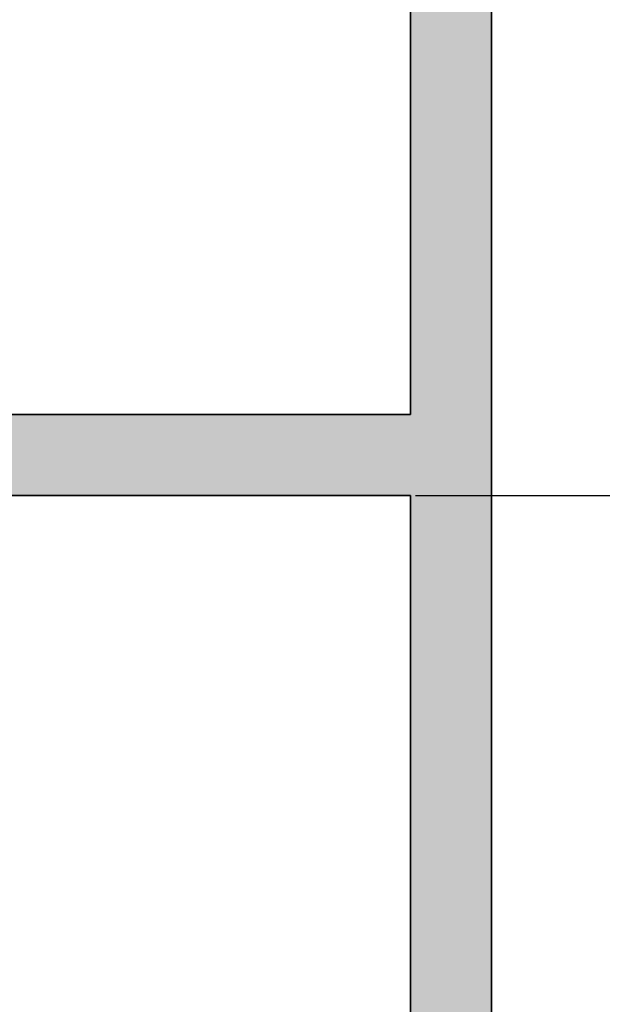
# Model space of a CAD drawing. Units: millimetres. Extents: x -22994 to 29398, y -19990 to 20176.
# Tile 38 of 135: x 183.3 to 190.48, y 41.76 to 53.9. Entities that reach past the tile are written whole.
import ezdxf
from ezdxf import colors
from ezdxf.entities.mleader import LeaderData, LeaderLine
from ezdxf.math import Vec2, Vec3

# ---------------------------------------------------------------- set-up
doc = ezdxf.new("R2010")
doc.units = ezdxf.units.MM
doc.header["$MEASUREMENT"] = 0
for name, color, linetype, lineweight in [('M-ANNO-TEXT', 7, 'Continuous', 25), ('M-DIMS', 2, 'Continuous', 18), ('M-EQPM-PATT', 7, 'Continuous', 18), ('M-PIPE', 7, 'Continuous', 35)]:
    doc.layers.add(name, color=color, linetype=linetype, lineweight=lineweight)
doc.styles.get("Standard").update_dxf_attribs({"font": 'arial.ttf'})
doc.dimstyles.get("Standard").update_dxf_attribs({"dimtxt": 0.18, "dimasz": 10000, "dimexe": 0.18, "dimexo": 0.0625, "dimgap": 0.09, "dimtad": 0, "dimtih": 1, "dimtoh": 1, "dimdec": 0, "dimzin": 0, "dimdsep": 46, "dimtxsty": 'Standard', "dimcen": 0.09, "dimadec": 0, "dimazin": 0, "dimtfac": 1, "dimtdec": 0, "dimtofl": 0, "dimtmove": 0, "dimatfit": 3, "dimfxl": 1, "dimtolj": 1, "dimtzin": 0, "dimlwd": 30, "dimarcsym": 0})

# ---------------------------------------------------------------- blocks, each defined once
blk = doc.blocks.new('*D2')
at = {"layer": 'Defpoints', "color": 0, "transparency": 16777216}
for p in [(6.677, 10.271), (290.852, 10.271), (290.852, -5.079)]:
    blk.add_point(p, dxfattribs=at)
at = {"layer": 'M-DIMS', "color": 0, "lineweight": -2, "transparency": 16777216}
for p, q in [((6.677, 10.209), (6.677, -5.259)), ((290.852, 10.209), (290.852, -5.259))]:
    blk.add_line(p, q, dxfattribs=at)
at = {"layer": 'M-DIMS', "color": 0, "lineweight": 30, "transparency": 16777216}
for p, q in [((-9993.323, -5.079), (-19993.323, -5.079)), ((10290.852, -5.079), (20290.852, -5.079))]:
    blk.add_line(p, q, dxfattribs=at)
at = {"layer": 'M-DIMS', "color": 0, "transparency": 16777216}
for points in [[(-9993.323, 1661.588), (-9993.323, -1671.745), (6.677, -5.079)], [(10290.852, 1661.588), (10290.852, -1671.745), (290.852, -5.079)]]:
    blk.add_solid(points, dxfattribs=at)
at = {"layer": 'M-DIMS', "color": 0, "transparency": 16777216, "insert": (148.765, -5.079), "char_height": 0.18, "attachment_point": 5}
blk.add_mtext('\\A1;284.2', dxfattribs=at)
blk = doc.blocks.new('*D3')
at = {"layer": 'Defpoints', "color": 0, "transparency": 16777216}
for p in [(110.265, 204.165), (110.265, 176.366), (95.833, 127.967)]:
    blk.add_point(p, dxfattribs=at)
at = {"layer": 'M-DIMS', "color": 0, "lineweight": -2, "transparency": 16777216}
for p, q in [((95.833, 128.03), (95.833, 204.345)), ((110.265, 176.429), (110.265, 204.345))]:
    blk.add_line(p, q, dxfattribs=at)
at = {"layer": 'M-DIMS', "color": 0, "lineweight": 30, "transparency": 16777216}
for p, q in [((-9904.167, 204.165), (-19904.167, 204.165)), ((10110.265, 204.165), (20110.265, 204.165))]:
    blk.add_line(p, q, dxfattribs=at)
at = {"layer": 'M-DIMS', "color": 0, "transparency": 16777216}
for points in [[(-9904.167, 1870.832), (-9904.167, -1462.501), (95.833, 204.165)], [(10110.265, 1870.832), (10110.265, -1462.501), (110.265, 204.165)]]:
    blk.add_solid(points, dxfattribs=at)
at = {"layer": 'M-DIMS', "color": 0, "transparency": 16777216, "insert": (103.049, 204.165), "char_height": 0.18, "attachment_point": 5}
blk.add_mtext('\\A1;14.432', dxfattribs=at)
blk = doc.blocks.new('*D4')
at = {"layer": 'Defpoints', "color": 0, "transparency": 16777216}
for p in [(116.265, 204.165), (110.265, 176.366), (116.265, 176.366)]:
    blk.add_point(p, dxfattribs=at)
at = {"layer": 'M-DIMS', "color": 0, "lineweight": -2, "transparency": 16777216}
for p, q in [((110.265, 176.429), (110.265, 204.345)), ((116.265, 176.429), (116.265, 204.345))]:
    blk.add_line(p, q, dxfattribs=at)
at = {"layer": 'M-DIMS', "color": 0, "lineweight": 30, "transparency": 16777216}
for p, q in [((-9889.735, 204.165), (-19889.735, 204.165)), ((10116.265, 204.165), (20116.265, 204.165))]:
    blk.add_line(p, q, dxfattribs=at)
at = {"layer": 'M-DIMS', "color": 0, "transparency": 16777216}
for points in [[(-9889.735, 1870.832), (-9889.735, -1462.501), (110.265, 204.165)], [(10116.265, 1870.832), (10116.265, -1462.501), (116.265, 204.165)]]:
    blk.add_solid(points, dxfattribs=at)
at = {"layer": 'M-DIMS', "color": 0, "transparency": 16777216, "insert": (113.265, 204.165), "char_height": 0.18, "attachment_point": 5}
blk.add_mtext('\\A1;6', dxfattribs=at)
blk = doc.blocks.new('*D5')
at = {"layer": 'Defpoints', "color": 0, "transparency": 16777216}
for p in [(181.265, 204.165), (116.265, 176.366), (181.265, 176.366)]:
    blk.add_point(p, dxfattribs=at)
at = {"layer": 'M-DIMS', "color": 0, "lineweight": -2, "transparency": 16777216}
for p, q in [((116.265, 176.429), (116.265, 204.345)), ((181.265, 176.429), (181.265, 204.345))]:
    blk.add_line(p, q, dxfattribs=at)
at = {"layer": 'M-DIMS', "color": 0, "lineweight": 30, "transparency": 16777216}
for p, q in [((-9883.735, 204.165), (-19883.735, 204.165)), ((10181.265, 204.165), (20181.265, 204.165))]:
    blk.add_line(p, q, dxfattribs=at)
at = {"layer": 'M-DIMS', "color": 0, "transparency": 16777216}
for points in [[(-9883.735, 1870.832), (-9883.735, -1462.501), (116.265, 204.165)], [(10181.265, 1870.832), (10181.265, -1462.501), (181.265, 204.165)]]:
    blk.add_solid(points, dxfattribs=at)
at = {"layer": 'M-DIMS', "color": 0, "transparency": 16777216, "insert": (148.765, 204.165), "char_height": 0.18, "attachment_point": 5}
blk.add_mtext('\\A1;65', dxfattribs=at)
blk = doc.blocks.new('*D6')
at = {"layer": 'Defpoints', "color": 0, "transparency": 16777216}
for p in [(187.265, 204.165), (181.265, 176.366), (187.265, 176.366)]:
    blk.add_point(p, dxfattribs=at)
at = {"layer": 'M-DIMS', "color": 0, "lineweight": -2, "transparency": 16777216}
for p, q in [((181.265, 176.429), (181.265, 204.345)), ((187.265, 176.429), (187.265, 204.345))]:
    blk.add_line(p, q, dxfattribs=at)
at = {"layer": 'M-DIMS', "color": 0, "lineweight": 30, "transparency": 16777216}
for p, q in [((-9818.735, 204.165), (-19818.735, 204.165)), ((10187.265, 204.165), (20187.265, 204.165))]:
    blk.add_line(p, q, dxfattribs=at)
at = {"layer": 'M-DIMS', "color": 0, "transparency": 16777216}
for points in [[(-9818.735, 1870.832), (-9818.735, -1462.501), (181.265, 204.165)], [(10187.265, 1870.832), (10187.265, -1462.501), (187.265, 204.165)]]:
    blk.add_solid(points, dxfattribs=at)
at = {"layer": 'M-DIMS', "color": 0, "transparency": 16777216, "insert": (184.265, 204.165), "char_height": 0.18, "attachment_point": 5}
blk.add_mtext('\\A1;6', dxfattribs=at)
blk = doc.blocks.new('*D7')
at = {"layer": 'Defpoints', "color": 0, "transparency": 16777216}
for p in [(201.697, 204.165), (187.265, 176.366), (201.697, 127.967)]:
    blk.add_point(p, dxfattribs=at)
at = {"layer": 'M-DIMS', "color": 0, "lineweight": -2, "transparency": 16777216}
for p, q in [((187.265, 176.429), (187.265, 204.345)), ((201.697, 128.03), (201.697, 204.345))]:
    blk.add_line(p, q, dxfattribs=at)
at = {"layer": 'M-DIMS', "color": 0, "lineweight": 30, "transparency": 16777216}
for p, q in [((-9812.735, 204.165), (-19812.735, 204.165)), ((10201.697, 204.165), (20201.697, 204.165))]:
    blk.add_line(p, q, dxfattribs=at)
at = {"layer": 'M-DIMS', "color": 0, "transparency": 16777216}
for points in [[(-9812.735, 1870.832), (-9812.735, -1462.501), (187.265, 204.165)], [(10201.697, 1870.832), (10201.697, -1462.501), (201.697, 204.165)]]:
    blk.add_solid(points, dxfattribs=at)
at = {"layer": 'M-DIMS', "color": 0, "transparency": 16777216, "insert": (194.481, 204.165), "char_height": 0.18, "attachment_point": 5}
blk.add_mtext('\\A1;14.432', dxfattribs=at)
blk = doc.blocks.new('*D8')
at = {"layer": 'Defpoints', "color": 0, "transparency": 16777216}
for p in [(227.648, 204.165), (227.648, 146.73), (201.697, 127.967)]:
    blk.add_point(p, dxfattribs=at)
at = {"layer": 'M-DIMS', "color": 0, "lineweight": -2, "transparency": 16777216}
for p, q in [((201.697, 128.03), (201.697, 204.345)), ((227.648, 146.792), (227.648, 204.345))]:
    blk.add_line(p, q, dxfattribs=at)
at = {"layer": 'M-DIMS', "color": 0, "lineweight": 30, "transparency": 16777216}
for p, q in [((-9798.303, 204.165), (-19798.303, 204.165)), ((10227.648, 204.165), (20227.648, 204.165))]:
    blk.add_line(p, q, dxfattribs=at)
at = {"layer": 'M-DIMS', "color": 0, "transparency": 16777216}
for points in [[(-9798.303, 1870.832), (-9798.303, -1462.501), (201.697, 204.165)], [(10227.648, 1870.832), (10227.648, -1462.501), (227.648, 204.165)]]:
    blk.add_solid(points, dxfattribs=at)
at = {"layer": 'M-DIMS', "color": 0, "transparency": 16777216, "insert": (214.673, 204.165), "char_height": 0.18, "attachment_point": 5}
blk.add_mtext('\\A1;25.95', dxfattribs=at)
blk = doc.blocks.new('*D9')
at = {"layer": 'Defpoints', "color": 0, "transparency": 16777216}
for p in [(187.265, 176.366), (306.202, 176.366), (290.852, 10.271)]:
    blk.add_point(p, dxfattribs=at)
at = {"layer": 'M-DIMS', "color": 0, "lineweight": 30, "transparency": 16777216}
for p, q in [((306.202, 10176.366), (306.202, 20176.366)), ((306.202, -9989.729), (306.202, -19989.729))]:
    blk.add_line(p, q, dxfattribs=at)
at = {"layer": 'M-DIMS', "color": 0, "lineweight": -2, "transparency": 16777216}
for p, q in [((187.327, 176.366), (306.382, 176.366)), ((290.915, 10.271), (306.382, 10.271))]:
    blk.add_line(p, q, dxfattribs=at)
at = {"layer": 'M-DIMS', "color": 0, "transparency": 16777216}
for points in [[(-1360.465, 10176.366), (1972.869, 10176.366), (306.202, 176.366)], [(-1360.465, -9989.729), (1972.869, -9989.729), (306.202, 10.271)]]:
    blk.add_solid(points, dxfattribs=at)
at = {"layer": 'M-DIMS', "color": 0, "transparency": 16777216, "insert": (306.202, 93.319), "char_height": 0.18, "attachment_point": 5}
blk.add_mtext('\\A1;166.1', dxfattribs=at)
blk = doc.blocks.new('*D10')
at = {"layer": 'Defpoints', "color": 0, "transparency": 16777216}
for p in [(125.65, 136.071), (133.346, 136.071), (133.346, -5.079)]:
    blk.add_point(p, dxfattribs=at)
at = {"layer": 'M-DIMS', "color": 0, "lineweight": -2, "transparency": 16777216}
for p, q in [((125.65, 136.009), (125.65, -5.259)), ((133.346, 136.009), (133.346, -5.259))]:
    blk.add_line(p, q, dxfattribs=at)
at = {"layer": 'M-DIMS', "color": 0, "lineweight": 30, "transparency": 16777216}
for p, q in [((-9874.35, -5.079), (-19874.35, -5.079)), ((10133.346, -5.079), (20133.346, -5.079))]:
    blk.add_line(p, q, dxfattribs=at)
at = {"layer": 'M-DIMS', "color": 0, "transparency": 16777216}
for points in [[(-9874.35, 1661.588), (-9874.35, -1671.745), (125.65, -5.079)], [(10133.346, 1661.588), (10133.346, -1671.745), (133.346, -5.079)]]:
    blk.add_solid(points, dxfattribs=at)
at = {"layer": 'M-DIMS', "color": 0, "transparency": 16777216, "insert": (129.498, -5.079), "char_height": 0.18, "attachment_point": 5}
blk.add_mtext('\\A1;7.696', dxfattribs=at)
blk = doc.blocks.new('*D11')
at = {"layer": 'Defpoints', "color": 0, "transparency": 16777216}
for p in [(133.346, 136.071), (135.65, 136.071), (135.65, -5.079)]:
    blk.add_point(p, dxfattribs=at)
at = {"layer": 'M-DIMS', "color": 0, "lineweight": -2, "transparency": 16777216}
for p, q in [((133.346, 136.009), (133.346, -5.259)), ((135.65, 136.009), (135.65, -5.259))]:
    blk.add_line(p, q, dxfattribs=at)
at = {"layer": 'M-DIMS', "color": 0, "lineweight": 30, "transparency": 16777216}
for p, q in [((-9866.654, -5.079), (-19866.654, -5.079)), ((10135.65, -5.079), (20135.65, -5.079))]:
    blk.add_line(p, q, dxfattribs=at)
at = {"layer": 'M-DIMS', "color": 0, "transparency": 16777216}
for points in [[(-9866.654, 1661.588), (-9866.654, -1671.745), (133.346, -5.079)], [(10135.65, 1661.588), (10135.65, -1671.745), (135.65, -5.079)]]:
    blk.add_solid(points, dxfattribs=at)
at = {"layer": 'M-DIMS', "color": 0, "transparency": 16777216, "insert": (134.498, -5.079), "char_height": 0.18, "attachment_point": 5}
blk.add_mtext('\\A1;2.304', dxfattribs=at)
blk = doc.blocks.new('*D12')
at = {"layer": 'Defpoints', "color": 0, "transparency": 16777216}
for p in [(135.65, 136.071), (145.65, 136.071), (145.65, -5.079)]:
    blk.add_point(p, dxfattribs=at)
at = {"layer": 'M-DIMS', "color": 0, "lineweight": -2, "transparency": 16777216}
for p, q in [((135.65, 136.009), (135.65, -5.259)), ((145.65, 136.009), (145.65, -5.259))]:
    blk.add_line(p, q, dxfattribs=at)
at = {"layer": 'M-DIMS', "color": 0, "lineweight": 30, "transparency": 16777216}
for p, q in [((-9864.35, -5.079), (-19864.35, -5.079)), ((10145.65, -5.079), (20145.65, -5.079))]:
    blk.add_line(p, q, dxfattribs=at)
at = {"layer": 'M-DIMS', "color": 0, "transparency": 16777216}
for points in [[(-9864.35, 1661.588), (-9864.35, -1671.745), (135.65, -5.079)], [(10145.65, 1661.588), (10145.65, -1671.745), (145.65, -5.079)]]:
    blk.add_solid(points, dxfattribs=at)
at = {"layer": 'M-DIMS', "color": 0, "transparency": 16777216, "insert": (140.65, -5.079), "char_height": 0.18, "attachment_point": 5}
blk.add_mtext('\\A1;10', dxfattribs=at)
blk = doc.blocks.new('*D13')
at = {"layer": 'Defpoints', "color": 0, "transparency": 16777216}
for p in [(145.65, 136.071), (155.65, 136.071), (155.65, -5.079)]:
    blk.add_point(p, dxfattribs=at)
at = {"layer": 'M-DIMS', "color": 0, "lineweight": -2, "transparency": 16777216}
for p, q in [((145.65, 136.009), (145.65, -5.259)), ((155.65, 136.009), (155.65, -5.259))]:
    blk.add_line(p, q, dxfattribs=at)
at = {"layer": 'M-DIMS', "color": 0, "lineweight": 30, "transparency": 16777216}
for p, q in [((-9854.35, -5.079), (-19854.35, -5.079)), ((10155.65, -5.079), (20155.65, -5.079))]:
    blk.add_line(p, q, dxfattribs=at)
at = {"layer": 'M-DIMS', "color": 0, "transparency": 16777216}
for points in [[(-9854.35, 1661.588), (-9854.35, -1671.745), (145.65, -5.079)], [(10155.65, 1661.588), (10155.65, -1671.745), (155.65, -5.079)]]:
    blk.add_solid(points, dxfattribs=at)
at = {"layer": 'M-DIMS', "color": 0, "transparency": 16777216, "insert": (150.65, -5.079), "char_height": 0.18, "attachment_point": 5}
blk.add_mtext('\\A1;10', dxfattribs=at)
blk = doc.blocks.new('*D14')
at = {"layer": 'Defpoints', "color": 0, "transparency": 16777216}
for p in [(155.65, 136.071), (165.65, 136.071), (165.65, -5.079)]:
    blk.add_point(p, dxfattribs=at)
at = {"layer": 'M-DIMS', "color": 0, "lineweight": -2, "transparency": 16777216}
for p, q in [((155.65, 136.009), (155.65, -5.259)), ((165.65, 136.009), (165.65, -5.259))]:
    blk.add_line(p, q, dxfattribs=at)
at = {"layer": 'M-DIMS', "color": 0, "lineweight": 30, "transparency": 16777216}
for p, q in [((-9844.35, -5.079), (-19844.35, -5.079)), ((10165.65, -5.079), (20165.65, -5.079))]:
    blk.add_line(p, q, dxfattribs=at)
at = {"layer": 'M-DIMS', "color": 0, "transparency": 16777216}
for points in [[(-9844.35, 1661.588), (-9844.35, -1671.745), (155.65, -5.079)], [(10165.65, 1661.588), (10165.65, -1671.745), (165.65, -5.079)]]:
    blk.add_solid(points, dxfattribs=at)
at = {"layer": 'M-DIMS', "color": 0, "transparency": 16777216, "insert": (160.65, -5.079), "char_height": 0.18, "attachment_point": 5}
blk.add_mtext('\\A1;10', dxfattribs=at)
blk = doc.blocks.new('*D15')
at = {"layer": 'Defpoints', "color": 0, "transparency": 16777216}
for p in [(173.346, 154.788), (173.346, 136.071), (306.202, 136.071)]:
    blk.add_point(p, dxfattribs=at)
at = {"layer": 'M-DIMS', "color": 0, "lineweight": 30, "transparency": 16777216}
for p, q in [((306.202, 10154.788), (306.202, 20154.788)), ((306.202, -9863.929), (306.202, -19863.929))]:
    blk.add_line(p, q, dxfattribs=at)
at = {"layer": 'M-DIMS', "color": 0, "lineweight": -2, "transparency": 16777216}
for p, q in [((173.408, 154.788), (306.382, 154.788)), ((173.408, 136.071), (306.382, 136.071))]:
    blk.add_line(p, q, dxfattribs=at)
at = {"layer": 'M-DIMS', "color": 0, "transparency": 16777216}
for points in [[(-1360.465, 10154.788), (1972.869, 10154.788), (306.202, 154.788)], [(-1360.465, -9863.929), (1972.869, -9863.929), (306.202, 136.071)]]:
    blk.add_solid(points, dxfattribs=at)
at = {"layer": 'M-DIMS', "color": 0, "transparency": 16777216, "insert": (306.202, 145.43), "char_height": 0.18, "attachment_point": 5}
blk.add_mtext('\\A1;18.717', dxfattribs=at)
blk = doc.blocks.new('*D16')
at = {"layer": 'Defpoints', "color": 0, "transparency": 16777216}
for p in [(120.17, 204.165), (110.466, 48.035), (120.17, 48.035)]:
    blk.add_point(p, dxfattribs=at)
at = {"layer": 'M-DIMS', "color": 0, "lineweight": -2, "transparency": 16777216}
for p, q in [((110.466, 48.097), (110.466, 204.345)), ((120.17, 48.097), (120.17, 204.345))]:
    blk.add_line(p, q, dxfattribs=at)
at = {"layer": 'M-DIMS', "color": 0, "lineweight": 30, "transparency": 16777216}
for p, q in [((-9889.534, 204.165), (-19889.534, 204.165)), ((10120.17, 204.165), (20120.17, 204.165))]:
    blk.add_line(p, q, dxfattribs=at)
at = {"layer": 'M-DIMS', "color": 0, "transparency": 16777216}
for points in [[(-9889.534, 1870.832), (-9889.534, -1462.501), (110.466, 204.165)], [(10120.17, 1870.832), (10120.17, -1462.501), (120.17, 204.165)]]:
    blk.add_solid(points, dxfattribs=at)
at = {"layer": 'M-DIMS', "color": 0, "transparency": 16777216, "insert": (115.318, 204.165), "char_height": 0.18, "attachment_point": 5}
blk.add_mtext('\\A1;9.704', dxfattribs=at)
blk = doc.blocks.new('*D17')
at = {"layer": 'Defpoints', "color": 0, "transparency": 16777216}
for p in [(126.17, 204.165), (120.17, 48.035), (126.17, 48.035)]:
    blk.add_point(p, dxfattribs=at)
at = {"layer": 'M-DIMS', "color": 0, "lineweight": -2, "transparency": 16777216}
for p, q in [((120.17, 48.097), (120.17, 204.345)), ((126.17, 48.097), (126.17, 204.345))]:
    blk.add_line(p, q, dxfattribs=at)
at = {"layer": 'M-DIMS', "color": 0, "lineweight": 30, "transparency": 16777216}
for p, q in [((-9879.83, 204.165), (-19879.83, 204.165)), ((10126.17, 204.165), (20126.17, 204.165))]:
    blk.add_line(p, q, dxfattribs=at)
at = {"layer": 'M-DIMS', "color": 0, "transparency": 16777216}
for points in [[(-9879.83, 1870.832), (-9879.83, -1462.501), (120.17, 204.165)], [(10126.17, 1870.832), (10126.17, -1462.501), (126.17, 204.165)]]:
    blk.add_solid(points, dxfattribs=at)
at = {"layer": 'M-DIMS', "color": 0, "transparency": 16777216, "insert": (123.17, 204.165), "char_height": 0.18, "attachment_point": 5}
blk.add_mtext('\\A1;6', dxfattribs=at)
blk = doc.blocks.new('*D18')
at = {"layer": 'Defpoints', "color": 0, "transparency": 16777216}
for p in [(132.17, 204.165), (126.17, 48.035), (132.17, 48.035)]:
    blk.add_point(p, dxfattribs=at)
at = {"layer": 'M-DIMS', "color": 0, "lineweight": -2, "transparency": 16777216}
for p, q in [((126.17, 48.097), (126.17, 204.345)), ((132.17, 48.097), (132.17, 204.345))]:
    blk.add_line(p, q, dxfattribs=at)
at = {"layer": 'M-DIMS', "color": 0, "lineweight": 30, "transparency": 16777216}
for p, q in [((-9873.83, 204.165), (-19873.83, 204.165)), ((10132.17, 204.165), (20132.17, 204.165))]:
    blk.add_line(p, q, dxfattribs=at)
at = {"layer": 'M-DIMS', "color": 0, "transparency": 16777216}
for points in [[(-9873.83, 1870.832), (-9873.83, -1462.501), (126.17, 204.165)], [(10132.17, 1870.832), (10132.17, -1462.501), (132.17, 204.165)]]:
    blk.add_solid(points, dxfattribs=at)
at = {"layer": 'M-DIMS', "color": 0, "transparency": 16777216, "insert": (129.17, 204.165), "char_height": 0.18, "attachment_point": 5}
blk.add_mtext('\\A1;6', dxfattribs=at)
blk = doc.blocks.new('*D19')
at = {"layer": 'Defpoints', "color": 0, "transparency": 16777216}
for p in [(138.17, 204.165), (132.17, 48.035), (138.17, 48.035)]:
    blk.add_point(p, dxfattribs=at)
at = {"layer": 'M-DIMS', "color": 0, "lineweight": -2, "transparency": 16777216}
for p, q in [((132.17, 48.097), (132.17, 204.345)), ((138.17, 48.097), (138.17, 204.345))]:
    blk.add_line(p, q, dxfattribs=at)
at = {"layer": 'M-DIMS', "color": 0, "lineweight": 30, "transparency": 16777216}
for p, q in [((-9867.83, 204.165), (-19867.83, 204.165)), ((10138.17, 204.165), (20138.17, 204.165))]:
    blk.add_line(p, q, dxfattribs=at)
at = {"layer": 'M-DIMS', "color": 0, "transparency": 16777216}
for points in [[(-9867.83, 1870.832), (-9867.83, -1462.501), (132.17, 204.165)], [(10138.17, 1870.832), (10138.17, -1462.501), (138.17, 204.165)]]:
    blk.add_solid(points, dxfattribs=at)
at = {"layer": 'M-DIMS', "color": 0, "transparency": 16777216, "insert": (135.17, 204.165), "char_height": 0.18, "attachment_point": 5}
blk.add_mtext('\\A1;6', dxfattribs=at)
blk = doc.blocks.new('*D20')
at = {"layer": 'Defpoints', "color": 0, "transparency": 16777216}
for p in [(144.17, 204.165), (138.17, 48.035), (144.17, 48.035)]:
    blk.add_point(p, dxfattribs=at)
at = {"layer": 'M-DIMS', "color": 0, "lineweight": -2, "transparency": 16777216}
for p, q in [((138.17, 48.097), (138.17, 204.345)), ((144.17, 48.097), (144.17, 204.345))]:
    blk.add_line(p, q, dxfattribs=at)
at = {"layer": 'M-DIMS', "color": 0, "lineweight": 30, "transparency": 16777216}
for p, q in [((-9861.83, 204.165), (-19861.83, 204.165)), ((10144.17, 204.165), (20144.17, 204.165))]:
    blk.add_line(p, q, dxfattribs=at)
at = {"layer": 'M-DIMS', "color": 0, "transparency": 16777216}
for points in [[(-9861.83, 1870.832), (-9861.83, -1462.501), (138.17, 204.165)], [(10144.17, 1870.832), (10144.17, -1462.501), (144.17, 204.165)]]:
    blk.add_solid(points, dxfattribs=at)
at = {"layer": 'M-DIMS', "color": 0, "transparency": 16777216, "insert": (141.17, 204.165), "char_height": 0.18, "attachment_point": 5}
blk.add_mtext('\\A1;6', dxfattribs=at)
blk = doc.blocks.new('*D21')
at = {"layer": 'Defpoints', "color": 0, "transparency": 16777216}
for p in [(149.116, 204.165), (144.17, 48.035), (149.116, 48.035)]:
    blk.add_point(p, dxfattribs=at)
at = {"layer": 'M-DIMS', "color": 0, "lineweight": -2, "transparency": 16777216}
for p, q in [((144.17, 48.097), (144.17, 204.345)), ((149.116, 48.097), (149.116, 204.345))]:
    blk.add_line(p, q, dxfattribs=at)
at = {"layer": 'M-DIMS', "color": 0, "lineweight": 30, "transparency": 16777216}
for p, q in [((-9855.83, 204.165), (-19855.83, 204.165)), ((10149.116, 204.165), (20149.116, 204.165))]:
    blk.add_line(p, q, dxfattribs=at)
at = {"layer": 'M-DIMS', "color": 0, "transparency": 16777216}
for points in [[(-9855.83, 1870.832), (-9855.83, -1462.501), (144.17, 204.165)], [(10149.116, 1870.832), (10149.116, -1462.501), (149.116, 204.165)]]:
    blk.add_solid(points, dxfattribs=at)
at = {"layer": 'M-DIMS', "color": 0, "transparency": 16777216, "insert": (146.643, 204.165), "char_height": 0.18, "attachment_point": 5}
blk.add_mtext('\\A1;4.945', dxfattribs=at)
blk = doc.blocks.new('*D22')
at = {"layer": 'Defpoints', "color": 0, "transparency": 16777216}
for p in [(149.116, 30.99), (155.116, 30.99), (155.116, -5.079)]:
    blk.add_point(p, dxfattribs=at)
at = {"layer": 'M-DIMS', "color": 0, "lineweight": -2, "transparency": 16777216}
for p, q in [((149.116, 30.927), (149.116, -5.259)), ((155.116, 30.927), (155.116, -5.259))]:
    blk.add_line(p, q, dxfattribs=at)
at = {"layer": 'M-DIMS', "color": 0, "lineweight": 30, "transparency": 16777216}
for p, q in [((-9850.884, -5.079), (-19850.884, -5.079)), ((10155.116, -5.079), (20155.116, -5.079))]:
    blk.add_line(p, q, dxfattribs=at)
at = {"layer": 'M-DIMS', "color": 0, "transparency": 16777216}
for points in [[(-9850.884, 1661.588), (-9850.884, -1671.745), (149.116, -5.079)], [(10155.116, 1661.588), (10155.116, -1671.745), (155.116, -5.079)]]:
    blk.add_solid(points, dxfattribs=at)
at = {"layer": 'M-DIMS', "color": 0, "transparency": 16777216, "insert": (152.116, -5.079), "char_height": 0.18, "attachment_point": 5}
blk.add_mtext('\\A1;6', dxfattribs=at)
blk = doc.blocks.new('*D23')
at = {"layer": 'Defpoints', "color": 0, "transparency": 16777216}
for p in [(155.116, 30.99), (161.116, 30.99), (161.116, -5.079)]:
    blk.add_point(p, dxfattribs=at)
at = {"layer": 'M-DIMS', "color": 0, "lineweight": -2, "transparency": 16777216}
for p, q in [((155.116, 30.927), (155.116, -5.259)), ((161.116, 30.927), (161.116, -5.259))]:
    blk.add_line(p, q, dxfattribs=at)
at = {"layer": 'M-DIMS', "color": 0, "lineweight": 30, "transparency": 16777216}
for p, q in [((-9844.884, -5.079), (-19844.884, -5.079)), ((10161.116, -5.079), (20161.116, -5.079))]:
    blk.add_line(p, q, dxfattribs=at)
at = {"layer": 'M-DIMS', "color": 0, "transparency": 16777216}
for points in [[(-9844.884, 1661.588), (-9844.884, -1671.745), (155.116, -5.079)], [(10161.116, 1661.588), (10161.116, -1671.745), (161.116, -5.079)]]:
    blk.add_solid(points, dxfattribs=at)
at = {"layer": 'M-DIMS', "color": 0, "transparency": 16777216, "insert": (158.116, -5.079), "char_height": 0.18, "attachment_point": 5}
blk.add_mtext('\\A1;6', dxfattribs=at)
blk = doc.blocks.new('*D24')
at = {"layer": 'Defpoints', "color": 0, "transparency": 16777216}
for p in [(161.116, 30.99), (166.439, 30.99), (166.439, -5.079)]:
    blk.add_point(p, dxfattribs=at)
at = {"layer": 'M-DIMS', "color": 0, "lineweight": -2, "transparency": 16777216}
for p, q in [((161.116, 30.927), (161.116, -5.259)), ((166.439, 30.927), (166.439, -5.259))]:
    blk.add_line(p, q, dxfattribs=at)
at = {"layer": 'M-DIMS', "color": 0, "lineweight": 30, "transparency": 16777216}
for p, q in [((-9838.884, -5.079), (-19838.884, -5.079)), ((10166.439, -5.079), (20166.439, -5.079))]:
    blk.add_line(p, q, dxfattribs=at)
at = {"layer": 'M-DIMS', "color": 0, "transparency": 16777216}
for points in [[(-9838.884, 1661.588), (-9838.884, -1671.745), (161.116, -5.079)], [(10166.439, 1661.588), (10166.439, -1671.745), (166.439, -5.079)]]:
    blk.add_solid(points, dxfattribs=at)
at = {"layer": 'M-DIMS', "color": 0, "transparency": 16777216, "insert": (163.777, -5.079), "char_height": 0.18, "attachment_point": 5}
blk.add_mtext('\\A1;5.323', dxfattribs=at)
blk = doc.blocks.new('*D25')
at = {"layer": 'Defpoints', "color": 0, "transparency": 16777216}
for p in [(166.439, 30.99), (172.439, 30.99), (172.439, -5.079)]:
    blk.add_point(p, dxfattribs=at)
at = {"layer": 'M-DIMS', "color": 0, "lineweight": -2, "transparency": 16777216}
for p, q in [((166.439, 30.927), (166.439, -5.259)), ((172.439, 30.927), (172.439, -5.259))]:
    blk.add_line(p, q, dxfattribs=at)
at = {"layer": 'M-DIMS', "color": 0, "lineweight": 30, "transparency": 16777216}
for p, q in [((-9833.561, -5.079), (-19833.561, -5.079)), ((10172.439, -5.079), (20172.439, -5.079))]:
    blk.add_line(p, q, dxfattribs=at)
at = {"layer": 'M-DIMS', "color": 0, "transparency": 16777216}
for points in [[(-9833.561, 1661.588), (-9833.561, -1671.745), (166.439, -5.079)], [(10172.439, 1661.588), (10172.439, -1671.745), (172.439, -5.079)]]:
    blk.add_solid(points, dxfattribs=at)
at = {"layer": 'M-DIMS', "color": 0, "transparency": 16777216, "insert": (169.439, -5.079), "char_height": 0.18, "attachment_point": 5}
blk.add_mtext('\\A1;6', dxfattribs=at)
blk = doc.blocks.new('*D26')
at = {"layer": 'Defpoints', "color": 0, "transparency": 16777216}
for p in [(172.439, 30.99), (178.439, 30.99), (178.439, -5.079)]:
    blk.add_point(p, dxfattribs=at)
at = {"layer": 'M-DIMS', "color": 0, "lineweight": -2, "transparency": 16777216}
for p, q in [((172.439, 30.927), (172.439, -5.259)), ((178.439, 30.927), (178.439, -5.259))]:
    blk.add_line(p, q, dxfattribs=at)
at = {"layer": 'M-DIMS', "color": 0, "lineweight": 30, "transparency": 16777216}
for p, q in [((-9827.561, -5.079), (-19827.561, -5.079)), ((10178.439, -5.079), (20178.439, -5.079))]:
    blk.add_line(p, q, dxfattribs=at)
at = {"layer": 'M-DIMS', "color": 0, "transparency": 16777216}
for points in [[(-9827.561, 1661.588), (-9827.561, -1671.745), (172.439, -5.079)], [(10178.439, 1661.588), (10178.439, -1671.745), (178.439, -5.079)]]:
    blk.add_solid(points, dxfattribs=at)
at = {"layer": 'M-DIMS', "color": 0, "transparency": 16777216, "insert": (175.439, -5.079), "char_height": 0.18, "attachment_point": 5}
blk.add_mtext('\\A1;6', dxfattribs=at)
blk = doc.blocks.new('*D27')
at = {"layer": 'Defpoints', "color": 0, "transparency": 16777216}
for p in [(178.439, 30.99), (188.117, 30.99), (188.117, -5.079)]:
    blk.add_point(p, dxfattribs=at)
at = {"layer": 'M-DIMS', "color": 0, "lineweight": -2, "transparency": 16777216}
for p, q in [((178.439, 30.927), (178.439, -5.259)), ((188.117, 30.927), (188.117, -5.259))]:
    blk.add_line(p, q, dxfattribs=at)
at = {"layer": 'M-DIMS', "color": 0, "lineweight": 30, "transparency": 16777216}
for p, q in [((-9821.561, -5.079), (-19821.561, -5.079)), ((10188.117, -5.079), (20188.117, -5.079))]:
    blk.add_line(p, q, dxfattribs=at)
at = {"layer": 'M-DIMS', "color": 0, "transparency": 16777216}
for points in [[(-9821.561, 1661.588), (-9821.561, -1671.745), (178.439, -5.079)], [(10188.117, 1661.588), (10188.117, -1671.745), (188.117, -5.079)]]:
    blk.add_solid(points, dxfattribs=at)
at = {"layer": 'M-DIMS', "color": 0, "transparency": 16777216, "insert": (183.278, -5.079), "char_height": 0.18, "attachment_point": 5}
blk.add_mtext('\\A1;9.679', dxfattribs=at)
blk = doc.blocks.new('*D28')
at = {"layer": 'Defpoints', "color": 0, "transparency": 16777216}
for p in [(188.117, 48.035), (306.202, 48.035), (188.117, 30.99)]:
    blk.add_point(p, dxfattribs=at)
at = {"layer": 'M-DIMS', "color": 0, "lineweight": 30, "transparency": 16777216}
for p, q in [((306.202, 10048.035), (306.202, 20048.035)), ((306.202, -9969.01), (306.202, -19969.01))]:
    blk.add_line(p, q, dxfattribs=at)
at = {"layer": 'M-DIMS', "color": 0, "lineweight": -2, "transparency": 16777216}
for p, q in [((188.18, 48.035), (306.382, 48.035)), ((188.18, 30.99), (306.382, 30.99))]:
    blk.add_line(p, q, dxfattribs=at)
at = {"layer": 'M-DIMS', "color": 0, "transparency": 16777216}
for points in [[(-1360.465, 10048.035), (1972.869, 10048.035), (306.202, 48.035)], [(-1360.465, -9969.01), (1972.869, -9969.01), (306.202, 30.99)]]:
    blk.add_solid(points, dxfattribs=at)
at = {"layer": 'M-DIMS', "color": 0, "transparency": 16777216, "insert": (306.202, 39.512), "char_height": 0.18, "attachment_point": 5}
blk.add_mtext('\\A1;17.045', dxfattribs=at)
blk = doc.blocks.new('*D29')
at = {"layer": 'Defpoints', "color": 0, "transparency": 16777216}
for p in [(36.801, 80.045), (64.03, 80.045)]:
    blk.add_point(p, dxfattribs=at)
at = {"layer": 'M-DIMS', "color": 0, "lineweight": -2, "transparency": 16777216}
for p, q in [((50.415, 79.955), (50.415, 80.135)), ((50.325, 80.045), (50.505, 80.045))]:
    blk.add_line(p, q, dxfattribs=at)
at = {"layer": 'M-DIMS', "color": 0, "lineweight": 30, "transparency": 16777216}
blk.add_line((20064.03, 80.03), (10064.03, 80.038), dxfattribs=at)
at = {"layer": 'M-DIMS', "color": 0, "transparency": 16777216}
blk.add_solid([(10064.031, 1746.704), (10064.028, -1586.629), (64.03, 80.045)], dxfattribs=at)
at = {"layer": 'M-DIMS', "color": 0, "transparency": 16777216, "insert": (20064.521, 80.03), "char_height": 0.18, "attachment_point": 5}
blk.add_mtext('\\A1;∅27.23', dxfattribs=at)
blk = doc.blocks.new('*D36')
at = {"layer": 'Defpoints', "color": 0, "transparency": 16777216}
for p in [(46.39, 31.303), (46.387, 26.593)]:
    blk.add_point(p, dxfattribs=at)
at = {"layer": 'M-DIMS', "color": 0, "lineweight": 30, "transparency": 16777216}
for p, q in [((57.15, 20031.301), (51.77, 10031.302)), ((10057.15, 20031.301), (57.15, 20031.301))]:
    blk.add_line(p, q, dxfattribs=at)
at = {"layer": 'M-DIMS', "color": 0, "lineweight": -2, "transparency": 16777216}
for p, q in [((46.389, 28.858), (46.389, 29.038)), ((46.299, 28.948), (46.479, 28.948))]:
    blk.add_line(p, q, dxfattribs=at)
at = {"layer": 'M-DIMS', "color": 0, "transparency": 16777216}
blk.add_solid([(-1614.896, 10032.199), (1718.436, 10030.405), (46.39, 31.303)], dxfattribs=at)
at = {"layer": 'M-DIMS', "color": 0, "transparency": 16777216, "insert": (10057.554, 20031.301), "char_height": 0.18, "attachment_point": 5}
blk.add_mtext('\\A1;∅4.71', dxfattribs=at)
blk = doc.blocks.new('*D37')
at = {"layer": 'Defpoints', "color": 0, "transparency": 16777216}
for p in [(54.834, 118.615), (59.494, 118.614)]:
    blk.add_point(p, dxfattribs=at)
at = {"layer": 'M-DIMS', "color": 0, "lineweight": -2, "transparency": 16777216}
for p, q in [((57.164, 118.524), (57.164, 118.704)), ((57.074, 118.614), (57.254, 118.614))]:
    blk.add_line(p, q, dxfattribs=at)
at = {"layer": 'M-DIMS', "color": 0, "lineweight": 30, "transparency": 16777216}
blk.add_line((20059.493, 116.253), (10059.494, 117.434), dxfattribs=at)
at = {"layer": 'M-DIMS', "color": 0, "transparency": 16777216}
blk.add_solid([(10059.69, 1784.1), (10059.297, -1549.233), (59.494, 118.614)], dxfattribs=at)
at = {"layer": 'M-DIMS', "color": 0, "transparency": 16777216, "insert": (20059.985, 116.253), "char_height": 0.18, "attachment_point": 5}
blk.add_mtext('\\A1;∅4.659', dxfattribs=at)

msp = doc.modelspace()

# ---------------------------------------------------------------- hatches: boundary and pattern name
at = {"layer": 'M-EQPM-PATT'}
h = msp.add_hatch(color=256, dxfattribs=at)
h.set_gradient(color1=(19, 155, 72), color2=(88, 186, 72), tint=1, name='CYLINDER')
h.paths.add_polyline_path([(109.4658, 29.9895), (189.1175, 29.9895), (189.1175, 77.6953), (128.1172, 77.6953, 0.4142136), (126.1172, 75.6953), (126.1172, 73.6953, 0.4142136), (128.1172, 71.6953), (178.5136, 71.6953, -0.4142136), (179.5136, 70.6953), (179.5136, 68.6953, -0.4142136), (178.5136, 67.6953), (128.1172, 67.6953, 0.4142136), (126.1172, 65.6953), (126.1172, 63.6953, 0.4142136), (128.1172, 61.6953), (178.5136, 61.6953, -0.4142136), (179.5136, 60.6953), (179.5136, 58.6953, -0.4142136), (178.5136, 57.6953), (109.7466, 57.6953, -0.4142136), (108.7466, 58.6953), (108.7466, 75.5922, 0.4142136), (106.7466, 77.5922), (101.8327, 77.5922), (101.8327, 76.5922), (106.7466, 76.5922, -0.4142136), (107.7466, 75.5922), (107.7466, 58.6953, 0.4142136), (109.7466, 56.6953), (178.5136, 56.6953, 0.4142136), (180.5136, 58.6953), (180.5136, 60.6953, 0.4142136), (178.5136, 62.6953), (128.1172, 62.6953, -0.4142136), (127.1172, 63.6953), (127.1172, 65.6953, -0.4142136), (128.1172, 66.6953), (178.5136, 66.6953, 0.4142136), (180.5136, 68.6953), (180.5136, 70.6953, 0.4142136), (178.5136, 72.6953), (128.1172, 72.6953, -0.4142136), (127.1172, 73.6953), (127.1172, 75.6953, -0.4142136), (128.1172, 76.6953), (188.1175, 76.6953), (188.1175, 49.0349), (110.4658, 49.0349), (110.4658, 51.9576), (101.8327, 51.9576), (101.8327, 50.9576), (109.4658, 50.9576), (109.4658, 48.5349)])
h.paths.add_polyline_path([(110.4658, 48.0349), (188.1175, 48.0349), (188.1175, 30.9895), (110.4658, 30.9895)], flags=16)
h.paths.add_polyline_path([(136.1519, 78.0082), (161.2406, 78.0082), (161.2406, 84.1903), (136.1519, 84.1903)], flags=9)

# ---------------------------------------------------------------- linework, layer by layer
at = {"layer": 'M-PIPE'}
for points in [[(189.1175, 29.9895), (189.1175, 77.6953), (128.1172, 77.6953, 0.4142136), (126.1172, 75.6953), (126.1172, 73.6953, 0.4142136), (128.1172, 71.6953), (178.5136, 71.6953, -0.4142136), (179.5136, 70.6953), (179.5136, 68.6953, -0.4142136), (178.5136, 67.6953), (128.1172, 67.6953, 0.4142136), (126.1172, 65.6953), (126.1172, 63.6953, 0.4142136), (128.1172, 61.6953), (178.5136, 61.6953, -0.4142136), (179.5136, 60.6953), (179.5136, 58.6953, -0.4142136), (178.5136, 57.6953), (109.7466, 57.6953, -0.4142136), (108.7466, 58.6953), (108.7466, 75.5922, 0.4142136), (106.7466, 77.5922), (101.8327, 77.5922)], [(188.1175, 49.0349), (188.1175, 76.6953), (128.1172, 76.6953, 0.4142136), (127.1172, 75.6953), (127.1172, 73.6953, 0.4142136), (128.1172, 72.6953), (178.5136, 72.6953, -0.4142136), (180.5136, 70.6953), (180.5136, 68.6953, -0.4142136), (178.5136, 66.6953), (128.1172, 66.6953, 0.4142136), (127.1172, 65.6953), (127.1172, 63.6953, 0.4142136), (128.1172, 62.6953), (178.5136, 62.6953, -0.4142136), (180.5136, 60.6953), (180.5136, 58.6953, -0.4142136), (178.5136, 56.6953), (109.7466, 56.6953, -0.4142136), (107.7466, 58.6953), (107.7466, 75.5922, 0.4142136), (106.7466, 76.5922), (101.8327, 76.5922)]]:
    msp.add_lwpolyline(points, format="xyb", dxfattribs=at)
for points in [[(110.4658, 49.0349), (188.1175, 49.0349)], [(188.1175, 30.9895), (110.4658, 30.9895), (110.4658, 48.0349), (188.1175, 48.0349)], [(188.1175, 30.9895), (188.1175, 48.0349)]]:
    msp.add_lwpolyline(points, dxfattribs=at)

# ---------------------------------------------------------------- dimensions: what is measured, and where the dimension line sits
at = {"layer": 'M-DIMS'}
for base, p1, p2, override, picture, middle in [((306.202, 176.3662), (290.852, 10.2713), (187.2647, 176.3662), {"dimdec": 1, "dimlfac": 1, "dimrnd": 0, "dimzin": 0, "dimdsep": 46, "dimlunit": 2}, '*D9', (306.202, 93.3187)), ((306.202, 136.0713), (173.3459, 154.788), (173.3459, 136.0713), {"dimdec": 3, "dimlfac": 1, "dimrnd": 0, "dimzin": 0, "dimdsep": 46, "dimlunit": 2}, '*D15', (306.202, 145.4297)), ((306.202, 48.0349), (188.1175, 30.9895), (188.1175, 48.0349), {"dimdec": 3, "dimlfac": 1, "dimrnd": 0, "dimzin": 0, "dimdsep": 46, "dimlunit": 2}, '*D28', (306.202, 39.5122))]:
    dim = msp.add_linear_dim(base=base, p1=p1, p2=p2, angle=90, dimstyle='Standard', override=override, dxfattribs=at)
    dim.commit()
    dim.dimension.update_dxf_attribs({"geometry": picture, "text_midpoint": middle})
dim = msp.add_diameter_dim_2p(p1=(46.3875, 26.5934), p2=(46.39, 31.3035), dimstyle='Standard', override={"dimdec": 2, "dimlfac": 1, "dimrnd": 0, "dimzin": 0, "dimdsep": 46, "dimlunit": 2}, dxfattribs=at)
dim.commit()
dim.dimension.update_dxf_attribs({"geometry": '*D36', "text_midpoint": (10057.5542, 20031.3006), "dimtype": 163})
for base, p1, p2, override, picture, middle in [((110.2647, 204.1654), (95.8327, 127.967), (110.2647, 176.3662), {"dimdec": 3, "dimlfac": 1, "dimrnd": 0, "dimzin": 0, "dimdsep": 46, "dimlunit": 2}, '*D3', (103.0487, 204.1654)), ((116.2647, 204.1654), (110.2647, 176.3662), (116.2647, 176.3662), {"dimdec": 0, "dimlfac": 1, "dimrnd": 0, "dimzin": 0, "dimdsep": 46, "dimlunit": 2}, '*D4', (113.2647, 204.1654)), ((120.1702, 204.1654), (110.4658, 48.0349), (120.1702, 48.0349), {"dimdec": 3, "dimlfac": 1, "dimrnd": 0, "dimzin": 0, "dimdsep": 46, "dimlunit": 2}, '*D16', (115.318, 204.1654)), ((181.2647, 204.1654), (116.2647, 176.3662), (181.2647, 176.3662), {"dimdec": 0, "dimlfac": 1, "dimrnd": 0, "dimzin": 0, "dimdsep": 46, "dimlunit": 2}, '*D5', (148.7647, 204.1654)), ((126.1702, 204.1654), (120.1702, 48.0349), (126.1702, 48.0349), {"dimdec": 0, "dimlfac": 1, "dimrnd": 0, "dimzin": 0, "dimdsep": 46, "dimlunit": 2}, '*D17', (123.1702, 204.1654)), ((132.1702, 204.1654), (126.1702, 48.0349), (132.1702, 48.0349), {"dimdec": 0, "dimlfac": 1, "dimrnd": 0, "dimzin": 0, "dimdsep": 46, "dimlunit": 2}, '*D18', (129.1702, 204.1654)), ((138.1702, 204.1654), (132.1702, 48.0349), (138.1702, 48.0349), {"dimdec": 0, "dimlfac": 1, "dimrnd": 0, "dimzin": 0, "dimdsep": 46, "dimlunit": 2}, '*D19', (135.1702, 204.1654)), ((144.1702, 204.1654), (138.1702, 48.0349), (144.1702, 48.0349), {"dimdec": 0, "dimlfac": 1, "dimrnd": 0, "dimzin": 0, "dimdsep": 46, "dimlunit": 2}, '*D20', (141.1702, 204.1654)), ((149.11567, 204.16539), (144.17023, 48.03494), (149.11567, 48.03494), {"dimdec": 3, "dimlfac": 1, "dimrnd": 0, "dimzin": 0, "dimdsep": 46, "dimlunit": 2}, '*D21', (146.64295, 204.16539)), ((187.2647, 204.1654), (181.2647, 176.3662), (187.2647, 176.3662), {"dimdec": 0, "dimlfac": 1, "dimrnd": 0, "dimzin": 0, "dimdsep": 46, "dimlunit": 2}, '*D6', (184.2647, 204.1654)), ((201.6967, 204.1654), (187.2647, 176.3662), (201.6967, 127.967), {"dimdec": 3, "dimlfac": 1, "dimrnd": 0, "dimzin": 0, "dimdsep": 46, "dimlunit": 2}, '*D7', (194.4807, 204.1654)), ((227.6485, 204.1654), (201.6967, 127.967), (227.6485, 146.7296), {"dimdec": 2, "dimlfac": 1, "dimrnd": 0, "dimzin": 0, "dimdsep": 46, "dimlunit": 2}, '*D8', (214.6726, 204.1654)), ((290.852, -5.0787), (6.6773, 10.2713), (290.852, 10.2713), {"dimdec": 1, "dimlfac": 1, "dimrnd": 0, "dimzin": 0, "dimdsep": 46, "dimlunit": 2}, '*D2', (148.7647, -5.0787)), ((133.3459, -5.0787), (125.6498, 136.0713), (133.3459, 136.0713), {"dimdec": 3, "dimlfac": 1, "dimrnd": 0, "dimzin": 0, "dimdsep": 46, "dimlunit": 2}, '*D10', (129.4978, -5.0787)), ((135.6498, -5.0787), (133.3459, 136.0713), (135.6498, 136.0713), {"dimdec": 3, "dimlfac": 1, "dimrnd": 0, "dimzin": 0, "dimdsep": 46, "dimlunit": 2}, '*D11', (134.4978, -5.0787)), ((145.6498, -5.0787), (135.6498, 136.0713), (145.6498, 136.0713), {"dimdec": 0, "dimlfac": 1, "dimrnd": 0, "dimzin": 0, "dimdsep": 46, "dimlunit": 2}, '*D12', (140.6498, -5.0787)), ((155.6498, -5.0787), (145.6498, 136.0713), (155.6498, 136.0713), {"dimdec": 0, "dimlfac": 1, "dimrnd": 0, "dimzin": 0, "dimdsep": 46, "dimlunit": 2}, '*D13', (150.6498, -5.0787)), ((155.1157, -5.0787), (149.1157, 30.9895), (155.1157, 30.9895), {"dimdec": 0, "dimlfac": 1, "dimrnd": 0, "dimzin": 0, "dimdsep": 46, "dimlunit": 2}, '*D22', (152.1157, -5.0787)), ((161.1157, -5.0787), (155.1157, 30.9895), (161.1157, 30.9895), {"dimdec": 0, "dimlfac": 1, "dimrnd": 0, "dimzin": 0, "dimdsep": 46, "dimlunit": 2}, '*D23', (158.1157, -5.0787)), ((165.6498, -5.0787), (155.6498, 136.0713), (165.6498, 136.0713), {"dimdec": 0, "dimlfac": 1, "dimrnd": 0, "dimzin": 0, "dimdsep": 46, "dimlunit": 2}, '*D14', (160.6498, -5.0787)), ((166.4387, -5.0787), (161.1157, 30.9895), (166.4387, 30.9895), {"dimdec": 3, "dimlfac": 1, "dimrnd": 0, "dimzin": 0, "dimdsep": 46, "dimlunit": 2}, '*D24', (163.7772, -5.0787)), ((172.4387, -5.0787), (166.4387, 30.9895), (172.4387, 30.9895), {"dimdec": 0, "dimlfac": 1, "dimrnd": 0, "dimzin": 0, "dimdsep": 46, "dimlunit": 2}, '*D25', (169.4387, -5.0787)), ((178.4387, -5.0787), (172.4387, 30.9895), (178.4387, 30.9895), {"dimdec": 0, "dimlfac": 1, "dimrnd": 0, "dimzin": 0, "dimdsep": 46, "dimlunit": 2}, '*D26', (175.4387, -5.0787)), ((188.1175, -5.0787), (178.4387, 30.9895), (188.1175, 30.9895), {"dimdec": 3, "dimlfac": 1, "dimrnd": 0, "dimzin": 0, "dimdsep": 46, "dimlunit": 2}, '*D27', (183.2781, -5.0787))]:
    dim = msp.add_linear_dim(base=base, p1=p1, p2=p2, dimstyle='Standard', override=override, dxfattribs=at)
    dim.commit()
    dim.dimension.update_dxf_attribs({"geometry": picture, "text_midpoint": middle})
for p1, p2, override, picture, middle in [((54.8343, 118.6145), (59.4936, 118.614), {"dimdec": 3, "dimlfac": 1, "dimrnd": 0, "dimzin": 0, "dimdsep": 46, "dimlunit": 2}, '*D37', (20059.4934, 116.2531)), ((36.8006, 80.045), (64.0296, 80.045), {"dimdec": 2, "dimlfac": 1, "dimrnd": 0, "dimzin": 0, "dimdsep": 46, "dimlunit": 2}, '*D29', (20064.0296, 80.0303))]:
    dim = msp.add_diameter_dim_2p(p1=p1, p2=p2, dimstyle='Standard', override=override, dxfattribs=at)
    dim.commit()
    dim.dimension.update_dxf_attribs({"geometry": picture, "text_midpoint": middle})

# ---------------------------------------------------------------- leaders
at = {"layer": 'M-ANNO-TEXT'}
ml = msp.add_multileader_mtext('Standard', dxfattribs=at)
ml.set_content('combustion chamber', color=256)
ml.set_leader_properties()
ml.build(insert=Vec2(0, 0))
ml.multileader.update_dxf_attribs({"dogleg_length": 0.36, "arrow_head_size": 200})
ctx = ml.context
ctx.base_point, ctx.char_height, ctx.arrow_head_size, ctx.landing_gap_size, ctx.plane_origin = Vec3(215.7321, 57.9149), 3, 200, 0.09, Vec3(189.1175, 57.9149)
notes = []
notes.append((ctx, [(0, (1, 1, 0), (215.3721, 57.9149), (1, 0), 0.36, [(0, [(189.1175, 57.9149)], 0, [])])]))
ctx.mtext.insert, ctx.mtext.flow_direction = Vec3(215.8221, 59.4394), 5
for ctx, leaders in notes:
    for number, flags, end, landing, length, lines in leaders:
        leader = LeaderData()
        leader.index, (leader.has_last_leader_line, leader.has_dogleg_vector, leader.attachment_direction) = number, flags
        leader.last_leader_point, leader.dogleg_vector, leader.dogleg_length = Vec3(end), Vec3(landing), length
        for number, points, colour, breaks in lines:
            line = LeaderLine()
            line.index, line.vertices, line.color, line.breaks = number, Vec3.list(points), colors.encode_raw_color(colour), breaks
            leader.lines.append(line)
        ctx.leaders.append(leader)

doc.saveas('drawing.dxf')
